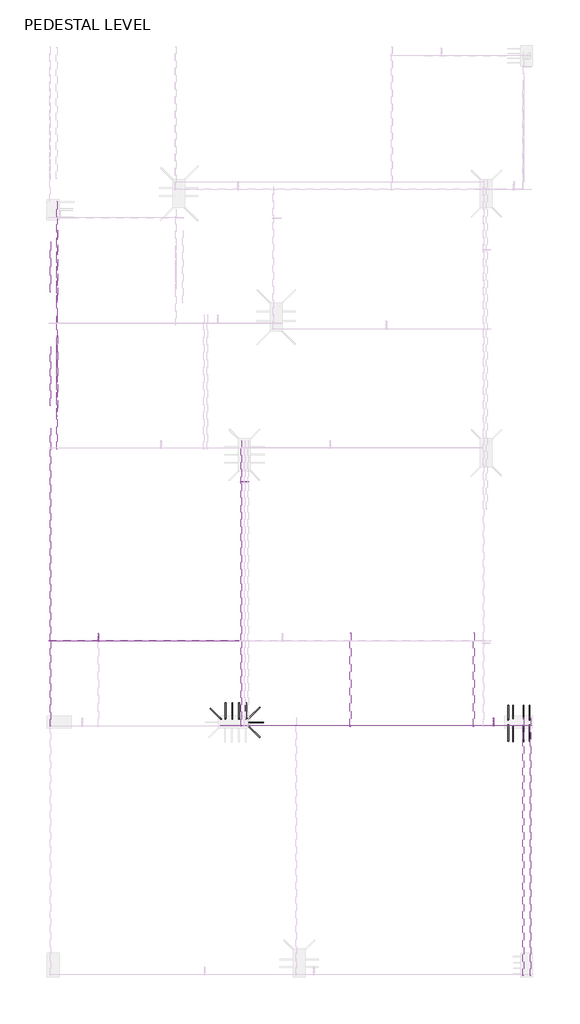
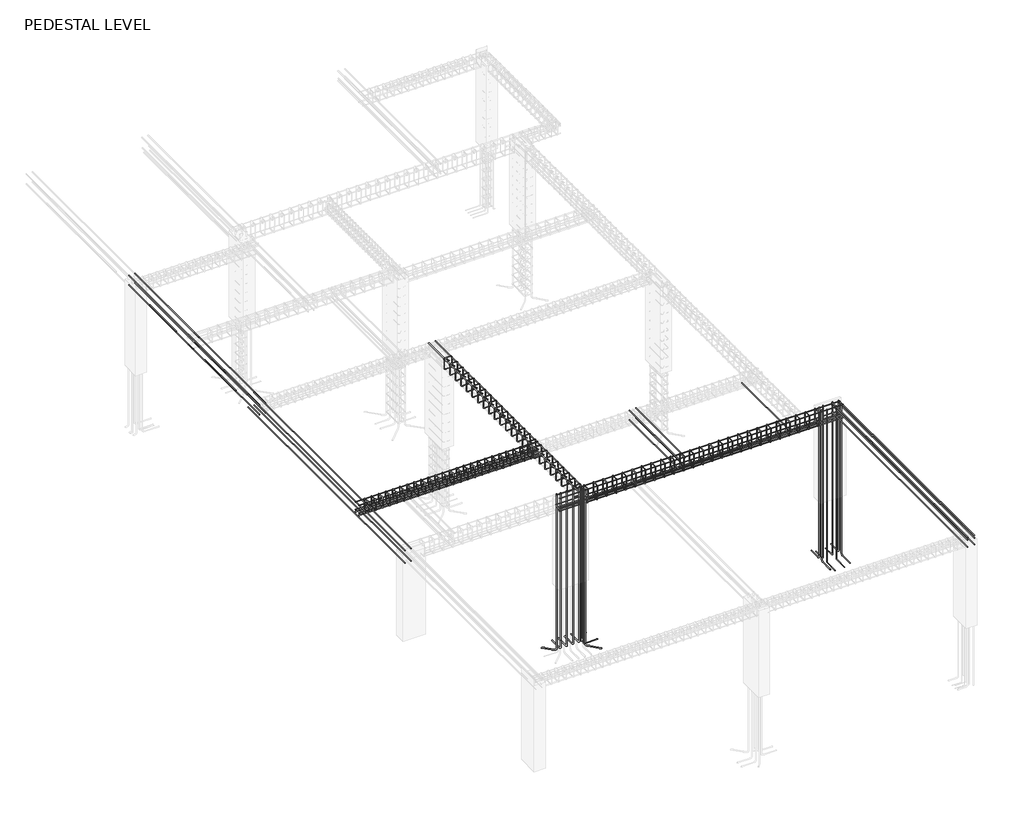
# One storey, part 3 of 8: 35 reinforcing bars.
"""IFC4 building model written with IfcOpenShell, lengths in millimetres."""

from ifc_helpers import new_model, si_unit, point, frame, origin, place, context, project, spatial, polyline, circle_curve, trimmed, segment, composite_curve, source, transform, mapped, element, save
from ifc_brep_helpers import swept_disk

model = new_model("IFC4")

# Units and contexts
model_context = context("Model", 3, world=origin())
ifc_project = project(units=[si_unit("LENGTHUNIT", "METRE", prefix="MILLI")], contexts=[model_context])

# Site, building, storey
site = spatial("IfcSite", under=ifc_project)
building = spatial("IfcBuilding", under=site)
storey = spatial("IfcBuildingStorey", under=building, Name="PEDESTAL LEVEL", Elevation=990.6)

# Reinforcing bars
placement = place(None, origin())
reinforcing_bar_shape = source(origin(), model_context, "Body", "SolidModel", [
    swept_disk(composite_curve([segment(polyline([(153625.7025689, -105009.8007776, 2960.0), (153625.7025689, -105009.8007776, -403.6)]), True, "CONTINUOUS"), segment(trimmed(circle_curve(frame((153625.7025689, -104969.8007776, -403.6), z_axis=(1.0, 0.0, 0.0), x_axis=(0.0, -40.0, 0.0)), 40.0), [point((153625.7025689, -105009.8007776, -403.6))], [point((153625.7025689, -104969.8007776, -443.6))], True, "CARTESIAN"), True, "CONTINUOUS"), segment(polyline([(153625.7025689, -104969.8007776, -443.6), (153625.7025689, -104708.6268212, -443.6)]), True, "CONTINUOUS")], self_intersect=False), 8.0),
])
element("IfcReinforcingBar", 1, at=placement, inside=storey, context=model_context, shape_type="MappedRepresentation", body=[
    mapped(reinforcing_bar_shape, transform((0.0, 0.0, 0.0), x_axis=(1.0, 0.0, 0.0), y_axis=(0.0, 1.0, 0.0), z_axis=(0.0, 0.0, 1.0))),
    mapped(reinforcing_bar_shape, transform((128.9768921, 0.0, 0.0), x_axis=(1.0, 0.0, 0.0), y_axis=(0.0, 1.0, 0.0), z_axis=(0.0, 0.0, 1.0))),
    mapped(reinforcing_bar_shape, transform((257.9537841, 0.0, 0.0), x_axis=(1.0, 0.0, 0.0), y_axis=(0.0, 1.0, 0.0), z_axis=(0.0, 0.0, 1.0))),
    mapped(reinforcing_bar_shape, transform((386.9306762, 0.0, 0.0), x_axis=(1.0, 0.0, 0.0), y_axis=(0.0, 1.0, 0.0), z_axis=(0.0, 0.0, 1.0))),
])
element("IfcReinforcingBar", 2, at=placement, inside=storey, context=model_context, shape_type="SolidModel", body=[
    swept_disk(composite_curve([segment(polyline([(153541.8370351, -105010.3572281, 2960.0), (153541.8370351, -105010.3572281, -403.6)]), True, "CONTINUOUS"), segment(trimmed(circle_curve(frame((153513.5527639, -104982.0729569, -403.6), z_axis=(0.7071067811865475, 0.7071067811865476, 0.0), x_axis=(28.28427120001288, -28.28427119999833, 0.0)), 40.0), [point((153541.8370351, -105010.3572281, -403.6))], [point((153513.5527639, -104982.0729569, -443.6))], True, "CARTESIAN"), True, "CONTINUOUS"), segment(polyline([(153513.5527639, -104982.0729569, -443.6), (153344.8044377, -104813.3246307, -443.6)]), True, "CONTINUOUS")], self_intersect=False), 8.0),
])
element("IfcReinforcingBar", 3, at=placement, inside=storey, context=model_context, shape_type="SolidModel", body=[
    swept_disk(composite_curve([segment(polyline([(154054.8805846, -105009.8007776, 2960.0), (154054.8805846, -105009.8007776, -403.6)]), True, "CONTINUOUS"), segment(trimmed(circle_curve(frame((154083.1648558, -104981.5165063, -403.6), z_axis=(0.7071067811865475, -0.7071067811865476, 0.0), x_axis=(-28.284271199983777, -28.28427129999909, 0.0)), 40.0), [point((154054.8805846, -105009.8007776, -403.6))], [point((154083.1648558, -104981.5165063, -443.6))], True, "CARTESIAN"), True, "CONTINUOUS"), segment(polyline([(154083.1648558, -104981.5165063, -443.6), (154270.4067315, -104794.2746307, -443.6)]), True, "CONTINUOUS")], self_intersect=False), 8.0),
])
element("IfcReinforcingBar", 4, at=placement, inside=storey, context=model_context, shape_type="SolidModel", body=[
    swept_disk(composite_curve([segment(polyline([(154054.3854805, -105141.9056735, 2960.0), (154054.3854805, -105141.9056735, -403.6)]), True, "CONTINUOUS"), segment(trimmed(circle_curve(frame((154082.6697518, -105170.1899448, -403.6), z_axis=(-0.7071067811865475, -0.7071067811865476, 0.0), x_axis=(-28.28427129998454, 28.28427129999909, 0.0)), 40.0), [point((154054.3854805, -105141.9056735, -403.6))], [point((154082.6697518, -105170.1899448, -443.6))], True, "CARTESIAN"), True, "CONTINUOUS"), segment(polyline([(154082.6697518, -105170.1899448, -443.6), (154270.4067315, -105357.9269245, -443.6)]), True, "CONTINUOUS")], self_intersect=False), 8.0),
])
element("IfcReinforcingBar", 5, at=placement, inside=storey, context=model_context, shape_type="SolidModel", body=[
    swept_disk(composite_curve([segment(polyline([(154058.8805846, -105076.4757776, 2960.0), (154058.8805846, -105076.4757776, -423.6)]), True, "CONTINUOUS"), segment(trimmed(circle_curve(frame((154078.8805846, -105076.4757776, -423.6), z_axis=(0.0, -1.0, 0.0), x_axis=(-20.0, 0.0, 0.0)), 20.0), [point((154058.8805846, -105076.4757776, -423.6))], [point((154078.8805846, -105076.4757776, -443.6))], True, "CARTESIAN"), True, "CONTINUOUS"), segment(polyline([(154078.8805846, -105076.4757776, -443.6), (154346.9805846, -105076.4757776, -443.6)]), True, "CONTINUOUS")], self_intersect=False), 4.0),
])
reinforcing_bar_2_shape = source(origin(), model_context, "Body", "SolidModel", [
    swept_disk(composite_curve([segment(polyline([(159353.7369154, -105125.7144861, 2970.0), (159353.7369154, -105125.7144861, -281.3228881)]), True, "CONTINUOUS"), segment(trimmed(circle_curve(frame((159353.7369154, -105165.7144861, -281.3228881), z_axis=(-1.0, 0.0, 0.0), x_axis=(0.0, 40.0, 0.0)), 40.0), [point((159353.7369154, -105125.7144861, -281.3228881))], [point((159353.7369154, -105165.7144861, -321.3228881))], True, "CARTESIAN"), True, "CONTINUOUS"), segment(polyline([(159353.7369154, -105165.7144861, -321.3228881), (159353.7369154, -105430.5144861, -321.3228881)]), True, "CONTINUOUS")], self_intersect=False), 8.0),
])
element("IfcReinforcingBar", 6, at=placement, inside=storey, context=model_context, shape_type="MappedRepresentation", body=[
    mapped(reinforcing_bar_2_shape, transform((0.0, 0.0, 0.0), x_axis=(1.0, 0.0, 0.0), y_axis=(0.0, 1.0, 0.0), z_axis=(0.0, 0.0, 1.0))),
    mapped(reinforcing_bar_2_shape, transform((-404.027417, 0.0, 0.0), x_axis=(1.0, 0.0, 0.0), y_axis=(0.0, 1.0, 0.0), z_axis=(0.0, 0.0, 1.0))),
])
reinforcing_bar_3_shape = source(origin(), model_context, "Body", "SolidModel", [
    swept_disk(composite_curve([segment(polyline([(159353.7369154, -105026.4870691, 2970.0), (159353.7369154, -105026.4870691, -278.4710053)]), True, "CONTINUOUS"), segment(trimmed(circle_curve(frame((159353.7369154, -104986.4870691, -278.4710053), z_axis=(1.0, 0.0, 0.0), x_axis=(0.0, -40.0, 0.0)), 40.0), [point((159353.7369154, -105026.4870691, -278.4710053))], [point((159353.7369154, -104986.4870691, -318.4710053))], True, "CARTESIAN"), True, "CONTINUOUS"), segment(polyline([(159353.7369154, -104986.4870691, -318.4710053), (159353.7369154, -104755.0681161, -318.4710053)]), True, "CONTINUOUS")], self_intersect=False), 8.0),
])
element("IfcReinforcingBar", 7, at=placement, inside=storey, context=model_context, shape_type="MappedRepresentation", body=[
    mapped(reinforcing_bar_3_shape, transform((0.0, 0.0, 0.0), x_axis=(1.0, 0.0, 0.0), y_axis=(0.0, 1.0, 0.0), z_axis=(0.0, 0.0, 1.0))),
    mapped(reinforcing_bar_3_shape, transform((-404.027417, 0.0, 0.0), x_axis=(1.0, 0.0, 0.0), y_axis=(0.0, 1.0, 0.0), z_axis=(0.0, 0.0, 1.0))),
])
reinforcing_bar_4_shape = source(origin(), model_context, "Body", "SolidModel", [
    swept_disk(composite_curve([segment(polyline([(159237.8663807, -105148.4007776, 2970.0), (159237.8663807, -105148.4007776, -348.4618667)]), True, "CONTINUOUS"), segment(trimmed(circle_curve(frame((159237.8663807, -105168.4007776, -348.4618667), z_axis=(-1.0, 0.0, 0.0), x_axis=(0.0, 20.0, 0.0)), 20.0), [point((159237.8663807, -105148.4007776, -348.4618667))], [point((159237.8663807, -105168.4007776, -368.4618667))], True, "CARTESIAN"), True, "CONTINUOUS"), segment(polyline([(159237.8663807, -105168.4007776, -368.4618667), (159237.8663807, -105442.4007776, -368.4618667)]), True, "CONTINUOUS")], self_intersect=False), 4.0),
])
element("IfcReinforcingBar", 8, at=placement, inside=storey, context=model_context, shape_type="MappedRepresentation", body=[
    mapped(reinforcing_bar_4_shape, transform((0.0, 0.0, 0.0), x_axis=(1.0, 0.0, 0.0), y_axis=(0.0, 1.0, 0.0), z_axis=(0.0, 0.0, 1.0))),
    mapped(reinforcing_bar_4_shape, transform((-197.0944443, 0.0, 0.0), x_axis=(1.0, 0.0, 0.0), y_axis=(0.0, 1.0, 0.0), z_axis=(0.0, 0.0, 1.0))),
])
reinforcing_bar_5_shape = source(origin(), model_context, "Body", "SolidModel", [
    swept_disk(composite_curve([segment(polyline([(159237.8663807, -105003.8007776, 2970.0), (159237.8663807, -105003.8007776, -348.4618667)]), True, "CONTINUOUS"), segment(trimmed(circle_curve(frame((159237.8663807, -104983.8007776, -348.4618667), z_axis=(1.0, 0.0, 0.0), x_axis=(0.0, -20.0, 0.0)), 20.0), [point((159237.8663807, -105003.8007776, -348.4618667))], [point((159237.8663807, -104983.8007776, -368.4618667))], True, "CARTESIAN"), True, "CONTINUOUS"), segment(polyline([(159237.8663807, -104983.8007776, -368.4618667), (159237.8663807, -104756.6548318, -368.4618667)]), True, "CONTINUOUS")], self_intersect=False), 4.0),
])
element("IfcReinforcingBar", 9, at=placement, inside=storey, context=model_context, shape_type="MappedRepresentation", body=[
    mapped(reinforcing_bar_5_shape, transform((0.0, 0.0, 0.0), x_axis=(1.0, 0.0, 0.0), y_axis=(0.0, 1.0, 0.0), z_axis=(0.0, 0.0, 1.0))),
    mapped(reinforcing_bar_5_shape, transform((-197.0944443, 0.0, 0.0), x_axis=(1.0, 0.0, 0.0), y_axis=(0.0, 1.0, 0.0), z_axis=(0.0, 0.0, 1.0))),
])
reinforcing_bar_6_shape = source(origin(), model_context, "Body", "SolidModel", [
    swept_disk(composite_curve([segment(polyline([(150331.3521391, -97578.5007776, 2953.0710678), (150331.3521391, -95276.3007776, 2953.0710678)]), True, "CONTINUOUS")], self_intersect=False), 6.0),
])
element("IfcReinforcingBar", 10, at=placement, inside=storey, context=model_context, shape_type="MappedRepresentation", body=[
    mapped(reinforcing_bar_6_shape, transform((0.0, 0.0, 0.0), x_axis=(1.0, 0.0, 0.0), y_axis=(0.0, 1.0, 0.0), z_axis=(0.0, 0.0, 1.0))),
    mapped(reinforcing_bar_6_shape, transform((124.7421356, 0.0, 0.0), x_axis=(1.0, 0.0, 0.0), y_axis=(0.0, 1.0, 0.0), z_axis=(0.0, 0.0, 1.0))),
])
reinforcing_bar_7_shape = source(origin(), model_context, "Body", "SolidModel", [
    swept_disk(composite_curve([segment(polyline([(150331.3521391, -97578.5007776, 2742.1289322), (150331.3521391, -95276.3007776, 2742.1289322)]), True, "CONTINUOUS")], self_intersect=False), 6.0),
])
element("IfcReinforcingBar", 11, at=placement, inside=storey, context=model_context, shape_type="MappedRepresentation", body=[
    mapped(reinforcing_bar_7_shape, transform((0.0, 0.0, 0.0), x_axis=(1.0, 0.0, 0.0), y_axis=(0.0, 1.0, 0.0), z_axis=(0.0, 0.0, 1.0))),
    mapped(reinforcing_bar_7_shape, transform((124.7421356, 0.0, 0.0), x_axis=(1.0, 0.0, 0.0), y_axis=(0.0, 1.0, 0.0), z_axis=(0.0, 0.0, 1.0))),
])
element("IfcReinforcingBar", 12, at=placement, inside=storey, context=model_context, shape_type="SolidModel", body=[
    swept_disk(composite_curve([segment(polyline([(150328.4232069, -96983.6572557, 2771.4), (150328.4232069, -96032.524691, 2771.4)]), True, "CONTINUOUS")], self_intersect=False), 6.0),
])
element("IfcReinforcingBar", 13, at=placement, inside=storey, context=model_context, shape_type="SolidModel", body=[
    swept_disk(composite_curve([segment(polyline([(150459.0232069, -97175.4075722, 2771.4), (150459.0232069, -95820.3079229, 2771.4)]), True, "CONTINUOUS")], self_intersect=False), 6.0),
])
reinforcing_bar_8_shape = source(origin(), model_context, "Body", "SolidModel", [
    swept_disk(composite_curve([segment(polyline([(150331.3521391, -99940.7007776, 2953.0710678), (150331.3521391, -97409.9007776, 2953.0710678)]), True, "CONTINUOUS")], self_intersect=False), 6.0),
])
element("IfcReinforcingBar", 14, at=placement, inside=storey, context=model_context, shape_type="MappedRepresentation", body=[
    mapped(reinforcing_bar_8_shape, transform((0.0, 0.0, 0.0), x_axis=(1.0, 0.0, 0.0), y_axis=(0.0, 1.0, 0.0), z_axis=(0.0, 0.0, 1.0))),
    mapped(reinforcing_bar_8_shape, transform((124.7421356, 0.0, 0.0), x_axis=(1.0, 0.0, 0.0), y_axis=(0.0, 1.0, 0.0), z_axis=(0.0, 0.0, 1.0))),
])
reinforcing_bar_9_shape = source(origin(), model_context, "Body", "SolidModel", [
    swept_disk(composite_curve([segment(polyline([(150331.3521391, -99940.7007776, 2742.1289322), (150331.3521391, -97409.9007776, 2742.1289322)]), True, "CONTINUOUS")], self_intersect=False), 6.0),
])
element("IfcReinforcingBar", 15, at=placement, inside=storey, context=model_context, shape_type="MappedRepresentation", body=[
    mapped(reinforcing_bar_9_shape, transform((0.0, 0.0, 0.0), x_axis=(1.0, 0.0, 0.0), y_axis=(0.0, 1.0, 0.0), z_axis=(0.0, 0.0, 1.0))),
    mapped(reinforcing_bar_9_shape, transform((124.7421356, 0.0, 0.0), x_axis=(1.0, 0.0, 0.0), y_axis=(0.0, 1.0, 0.0), z_axis=(0.0, 0.0, 1.0))),
])
element("IfcReinforcingBar", 16, at=placement, inside=storey, context=model_context, shape_type="SolidModel", body=[
    swept_disk(composite_curve([segment(polyline([(150328.4232069, -99117.2572557, 2771.4), (150328.4232069, -98013.7246916, 2771.4)]), True, "CONTINUOUS")], self_intersect=False), 6.0),
])
element("IfcReinforcingBar", 17, at=placement, inside=storey, context=model_context, shape_type="SolidModel", body=[
    swept_disk(composite_curve([segment(polyline([(150459.0232069, -99316.7901782, 2771.4), (150459.0232069, -97803.9257644, 2771.4)]), True, "CONTINUOUS")], self_intersect=False), 6.0),
])
reinforcing_bar_10_shape = source(origin(), model_context, "Body", "SolidModel", [
    swept_disk(composite_curve([segment(polyline([(159236.7521391, -109846.7007776, 2953.0710678), (159236.7521391, -104991.8007776, 2953.0710678)]), True, "CONTINUOUS")], self_intersect=False), 6.0),
])
element("IfcReinforcingBar", 18, at=placement, inside=storey, context=model_context, shape_type="MappedRepresentation", body=[
    mapped(reinforcing_bar_10_shape, transform((0.0, 0.0, 0.0), x_axis=(1.0, 0.0, 0.0), y_axis=(0.0, 1.0, 0.0), z_axis=(0.0, 0.0, 1.0))),
    mapped(reinforcing_bar_10_shape, transform((134.7421356, 0.0, 0.0), x_axis=(1.0, 0.0, 0.0), y_axis=(0.0, 1.0, 0.0), z_axis=(0.0, 0.0, 1.0))),
])
reinforcing_bar_11_shape = source(origin(), model_context, "Body", "SolidModel", [
    swept_disk(composite_curve([segment(polyline([(159374.4232069, -109846.7007776, 2749.2), (159374.4232069, -104991.8007776, 2749.2)]), True, "CONTINUOUS")], self_intersect=False), 6.0),
])
element("IfcReinforcingBar", 19, at=placement, inside=storey, context=model_context, shape_type="MappedRepresentation", body=[
    mapped(reinforcing_bar_11_shape, transform((0.0, 0.0, 0.0), x_axis=(1.0, 0.0, 0.0), y_axis=(0.0, 1.0, 0.0), z_axis=(0.0, 0.0, 1.0))),
    mapped(reinforcing_bar_11_shape, transform((-140.6, 0.0, 0.0), x_axis=(1.0, 0.0, 0.0), y_axis=(0.0, 1.0, 0.0), z_axis=(0.0, 0.0, 1.0))),
])
reinforcing_bar_12_shape = source(origin(), model_context, "Body", "SolidModel", [
    swept_disk(composite_curve([segment(polyline([(159233.8232069, -109846.7007776, 2896.5439131), (159233.8232069, -104991.8007776, 2896.5439131)]), True, "CONTINUOUS")], self_intersect=False), 6.0),
])
element("IfcReinforcingBar", 20, at=placement, inside=storey, context=model_context, shape_type="MappedRepresentation", body=[
    mapped(reinforcing_bar_12_shape, transform((0.0, 0.0, 0.0), x_axis=(1.0, 0.0, 0.0), y_axis=(0.0, 1.0, 0.0), z_axis=(0.0, 0.0, 1.0))),
    mapped(reinforcing_bar_12_shape, transform((140.6, 0.0, 0.0), x_axis=(1.0, 0.0, 0.0), y_axis=(0.0, 1.0, 0.0), z_axis=(0.0, 0.0, 1.0))),
])
reinforcing_bar_13_shape = source(origin(), model_context, "Body", "SolidModel", [
    swept_disk(composite_curve([segment(polyline([(150507.0232063, -103455.5119243, 2895.7954185), (150507.0232063, -103519.8586414, 2960.1421356)]), True, "CONTINUOUS"), segment(trimmed(circle_curve(frame((150507.0232063, -103534.000777, 2946.0), z_axis=(1.0, 0.0, 0.0), x_axis=(0.0, 14.142135599991889, 14.142135600000074)), 20.0), [point((150507.0232063, -103519.8586414, 2960.1421356))], [point((150507.0232063, -103554.000777, 2946.0))], True, "CARTESIAN"), True, "CONTINUOUS"), segment(polyline([(150507.0232063, -103554.000777, 2946.0), (150507.0232063, -103554.000777, 2749.2)]), True, "CONTINUOUS"), segment(trimmed(circle_curve(frame((150507.0232063, -103534.000777, 2749.2), z_axis=(1.0, 0.0, 0.0), x_axis=(0.0, -20.0, 0.0)), 20.0), [point((150507.0232063, -103554.000777, 2749.2))], [point((150507.0232063, -103534.000777, 2729.2))], True, "CARTESIAN"), True, "CONTINUOUS"), segment(polyline([(150507.0232063, -103534.000777, 2729.2), (150507.0232063, -103423.400777, 2729.2)]), True, "CONTINUOUS"), segment(trimmed(circle_curve(frame((150506.3479159, -103423.400777, 2749.1885963), z_axis=(0.9994298160123042, 0.0, 0.033764520811226544), x_axis=(0.6752903999877162, 0.0, -19.988596300000154)), 20.0), [point((150507.0232063, -103423.400777, 2729.2))], [point((150506.3479159, -103403.400777, 2749.1885963))], True, "CARTESIAN"), True, "CONTINUOUS"), segment(polyline([(150506.3479159, -103403.400777, 2749.1885963), (150499.6984967, -103403.400777, 2946.0114037)]), True, "CONTINUOUS"), segment(trimmed(circle_curve(frame((150499.6984967, -103423.400777, 2946.0114037), z_axis=(0.9994298160123042, 0.0, 0.033764520811226544), x_axis=(0.0, 20.0, 0.0)), 20.0), [point((150499.6984967, -103403.400777, 2946.0114037))], [point((150499.0232063, -103423.400777, 2966.0))], True, "CARTESIAN"), True, "CONTINUOUS"), segment(polyline([(150499.0232063, -103423.400777, 2966.0), (150499.0232063, -103534.000777, 2966.0)]), True, "CONTINUOUS"), segment(trimmed(circle_curve(frame((150499.0232063, -103534.000777, 2946.0), z_axis=(1.0, 0.0, 0.0), x_axis=(0.0, 0.0, 20.0)), 20.0), [point((150499.0232063, -103534.000777, 2966.0))], [point((150499.0232063, -103548.1429126, 2931.8578644))], True, "CARTESIAN"), True, "CONTINUOUS"), segment(polyline([(150499.0232063, -103548.1429126, 2931.8578644), (150499.0232063, -103483.7961955, 2867.5111473)]), True, "CONTINUOUS")], self_intersect=False), 4.0),
])
element("IfcReinforcingBar", 21, at=placement, inside=storey, context=model_context, shape_type="MappedRepresentation", body=[
    mapped(reinforcing_bar_13_shape, transform((0.0, 0.0, 0.0), x_axis=(1.0, 0.0, 0.0), y_axis=(0.0, 1.0, 0.0), z_axis=(0.0, 0.0, 1.0))),
    mapped(reinforcing_bar_13_shape, transform((146.2285817, 0.0, 0.0), x_axis=(1.0, 0.0, 0.0), y_axis=(0.0, 1.0, 0.0), z_axis=(0.0, 0.0, 1.0))),
    mapped(reinforcing_bar_13_shape, transform((292.4571634, 0.0, 0.0), x_axis=(1.0, 0.0, 0.0), y_axis=(0.0, 1.0, 0.0), z_axis=(0.0, 0.0, 1.0))),
    mapped(reinforcing_bar_13_shape, transform((438.6857451, 0.0, 0.0), x_axis=(1.0, 0.0, 0.0), y_axis=(0.0, 1.0, 0.0), z_axis=(0.0, 0.0, 1.0))),
    mapped(reinforcing_bar_13_shape, transform((584.9143268, 0.0, 0.0), x_axis=(1.0, 0.0, 0.0), y_axis=(0.0, 1.0, 0.0), z_axis=(0.0, 0.0, 1.0))),
    mapped(reinforcing_bar_13_shape, transform((731.1429084, 0.0, 0.0), x_axis=(1.0, 0.0, 0.0), y_axis=(0.0, 1.0, 0.0), z_axis=(0.0, 0.0, 1.0))),
    mapped(reinforcing_bar_13_shape, transform((877.3714901, 0.0, 0.0), x_axis=(1.0, 0.0, 0.0), y_axis=(0.0, 1.0, 0.0), z_axis=(0.0, 0.0, 1.0))),
    mapped(reinforcing_bar_13_shape, transform((1023.6000718, 0.0, 0.0), x_axis=(1.0, 0.0, 0.0), y_axis=(0.0, 1.0, 0.0), z_axis=(0.0, 0.0, 1.0))),
    mapped(reinforcing_bar_13_shape, transform((1169.8286535, 0.0, 0.0), x_axis=(1.0, 0.0, 0.0), y_axis=(0.0, 1.0, 0.0), z_axis=(0.0, 0.0, 1.0))),
    mapped(reinforcing_bar_13_shape, transform((1316.0572352, 0.0, 0.0), x_axis=(1.0, 0.0, 0.0), y_axis=(0.0, 1.0, 0.0), z_axis=(0.0, 0.0, 1.0))),
    mapped(reinforcing_bar_13_shape, transform((1462.2858169, 0.0, 0.0), x_axis=(1.0, 0.0, 0.0), y_axis=(0.0, 1.0, 0.0), z_axis=(0.0, 0.0, 1.0))),
    mapped(reinforcing_bar_13_shape, transform((1608.5143986, 0.0, 0.0), x_axis=(1.0, 0.0, 0.0), y_axis=(0.0, 1.0, 0.0), z_axis=(0.0, 0.0, 1.0))),
    mapped(reinforcing_bar_13_shape, transform((1754.7429803, 0.0, 0.0), x_axis=(1.0, 0.0, 0.0), y_axis=(0.0, 1.0, 0.0), z_axis=(0.0, 0.0, 1.0))),
    mapped(reinforcing_bar_13_shape, transform((1900.971562, 0.0, 0.0), x_axis=(1.0, 0.0, 0.0), y_axis=(0.0, 1.0, 0.0), z_axis=(0.0, 0.0, 1.0))),
    mapped(reinforcing_bar_13_shape, transform((2047.2001437, 0.0, 0.0), x_axis=(1.0, 0.0, 0.0), y_axis=(0.0, 1.0, 0.0), z_axis=(0.0, 0.0, 1.0))),
    mapped(reinforcing_bar_13_shape, transform((2193.4287253, 0.0, 0.0), x_axis=(1.0, 0.0, 0.0), y_axis=(0.0, 1.0, 0.0), z_axis=(0.0, 0.0, 1.0))),
    mapped(reinforcing_bar_13_shape, transform((2339.657307, 0.0, 0.0), x_axis=(1.0, 0.0, 0.0), y_axis=(0.0, 1.0, 0.0), z_axis=(0.0, 0.0, 1.0))),
    mapped(reinforcing_bar_13_shape, transform((2485.8858887, 0.0, 0.0), x_axis=(1.0, 0.0, 0.0), y_axis=(0.0, 1.0, 0.0), z_axis=(0.0, 0.0, 1.0))),
    mapped(reinforcing_bar_13_shape, transform((2632.1144704, 0.0, 0.0), x_axis=(1.0, 0.0, 0.0), y_axis=(0.0, 1.0, 0.0), z_axis=(0.0, 0.0, 1.0))),
    mapped(reinforcing_bar_13_shape, transform((2778.3430521, 0.0, 0.0), x_axis=(1.0, 0.0, 0.0), y_axis=(0.0, 1.0, 0.0), z_axis=(0.0, 0.0, 1.0))),
    mapped(reinforcing_bar_13_shape, transform((2924.5716338, 0.0, 0.0), x_axis=(1.0, 0.0, 0.0), y_axis=(0.0, 1.0, 0.0), z_axis=(0.0, 0.0, 1.0))),
    mapped(reinforcing_bar_13_shape, transform((3070.8002155, 0.0, 0.0), x_axis=(1.0, 0.0, 0.0), y_axis=(0.0, 1.0, 0.0), z_axis=(0.0, 0.0, 1.0))),
    mapped(reinforcing_bar_13_shape, transform((3217.0287972, 0.0, 0.0), x_axis=(1.0, 0.0, 0.0), y_axis=(0.0, 1.0, 0.0), z_axis=(0.0, 0.0, 1.0))),
    mapped(reinforcing_bar_13_shape, transform((3363.2573789, 0.0, 0.0), x_axis=(1.0, 0.0, 0.0), y_axis=(0.0, 1.0, 0.0), z_axis=(0.0, 0.0, 1.0))),
])
reinforcing_bar_14_shape = source(origin(), model_context, "Body", "SolidModel", [
    swept_disk(composite_curve([segment(polyline([(150304.4232069, -103416.3297092, 2953.0710678), (154072.8805846, -103416.3297092, 2953.0710678)]), True, "CONTINUOUS")], self_intersect=False), 6.0),
])
element("IfcReinforcingBar", 22, at=placement, inside=storey, context=model_context, shape_type="MappedRepresentation", body=[
    mapped(reinforcing_bar_14_shape, transform((0.0, 0.0, 0.0), x_axis=(1.0, 0.0, 0.0), y_axis=(0.0, 1.0, 0.0), z_axis=(0.0, 0.0, 1.0))),
    mapped(reinforcing_bar_14_shape, transform((0.0, -124.7421356, 0.0), x_axis=(1.0, 0.0, 0.0), y_axis=(0.0, 1.0, 0.0), z_axis=(0.0, 0.0, 1.0))),
])
reinforcing_bar_15_shape = source(origin(), model_context, "Body", "SolidModel", [
    swept_disk(composite_curve([segment(polyline([(150304.4232069, -103541.0718448, 2742.1289322), (154072.8805846, -103541.0718448, 2742.1289322)]), True, "CONTINUOUS")], self_intersect=False), 6.0),
])
element("IfcReinforcingBar", 23, at=placement, inside=storey, context=model_context, shape_type="MappedRepresentation", body=[
    mapped(reinforcing_bar_15_shape, transform((0.0, 0.0, 0.0), x_axis=(1.0, 0.0, 0.0), y_axis=(0.0, 1.0, 0.0), z_axis=(0.0, 0.0, 1.0))),
    mapped(reinforcing_bar_15_shape, transform((0.0, 124.7421356, 0.0), x_axis=(1.0, 0.0, 0.0), y_axis=(0.0, 1.0, 0.0), z_axis=(0.0, 0.0, 1.0))),
])
reinforcing_bar_16_shape = source(origin(), model_context, "Body", "SolidModel", [
    swept_disk(composite_curve([segment(polyline([(150304.4232069, -103544.000777, 2791.7182247), (154072.8805846, -103544.000777, 2791.7182247)]), True, "CONTINUOUS")], self_intersect=False), 6.0),
])
element("IfcReinforcingBar", 24, at=placement, inside=storey, context=model_context, shape_type="MappedRepresentation", body=[
    mapped(reinforcing_bar_16_shape, transform((0.0, 0.0, 0.0), x_axis=(1.0, 0.0, 0.0), y_axis=(0.0, 1.0, 0.0), z_axis=(0.0, 0.0, 1.0))),
    mapped(reinforcing_bar_16_shape, transform((0.0, 127.6710678, 0.0), x_axis=(1.0, 0.0, 0.0), y_axis=(0.0, 1.0, 0.0), z_axis=(0.0, 0.0, 1.0))),
])
reinforcing_bar_17_shape = source(origin(), model_context, "Body", "SolidModel", [
    swept_disk(composite_curve([segment(polyline([(150331.3521391, -105150.4007776, 2943.0710678), (150331.3521391, -99543.5007776, 2943.0710678)]), True, "CONTINUOUS")], self_intersect=False), 6.0),
])
element("IfcReinforcingBar", 25, at=placement, inside=storey, context=model_context, shape_type="MappedRepresentation", body=[
    mapped(reinforcing_bar_17_shape, transform((0.0, 0.0, 0.0), x_axis=(1.0, 0.0, 0.0), y_axis=(0.0, 1.0, 0.0), z_axis=(0.0, 0.0, 1.0))),
    mapped(reinforcing_bar_17_shape, transform((124.7421356, 0.0, 0.0), x_axis=(1.0, 0.0, 0.0), y_axis=(0.0, 1.0, 0.0), z_axis=(0.0, 0.0, 1.0))),
])
reinforcing_bar_18_shape = source(origin(), model_context, "Body", "SolidModel", [
    swept_disk(composite_curve([segment(polyline([(150331.3521391, -105150.4007776, 2665.826012), (150331.3521391, -99543.5007776, 2665.826012)]), True, "CONTINUOUS")], self_intersect=False), 6.0),
])
element("IfcReinforcingBar", 26, at=placement, inside=storey, context=model_context, shape_type="MappedRepresentation", body=[
    mapped(reinforcing_bar_18_shape, transform((0.0, 0.0, 0.0), x_axis=(1.0, 0.0, 0.0), y_axis=(0.0, 1.0, 0.0), z_axis=(0.0, 0.0, 1.0))),
    mapped(reinforcing_bar_18_shape, transform((124.7421356, 0.0, 0.0), x_axis=(1.0, 0.0, 0.0), y_axis=(0.0, 1.0, 0.0), z_axis=(0.0, 0.0, 1.0))),
])
reinforcing_bar_19_shape = source(origin(), model_context, "Body", "SolidModel", [
    swept_disk(composite_curve([segment(polyline([(154006.7694373, -100357.7007776, 2895.7954185), (153942.4227202, -100357.7007776, 2960.1421356)]), True, "CONTINUOUS"), segment(trimmed(circle_curve(frame((153928.2805846, -100357.7007776, 2946.0), z_axis=(0.0, -1.0, 0.0), x_axis=(14.14213560000644, 0.0, 14.142135600000074)), 20.0), [point((153942.4227202, -100357.7007776, 2960.1421356))], [point((153908.2805846, -100357.7007776, 2946.0))], True, "CARTESIAN"), True, "CONTINUOUS"), segment(polyline([(153908.2805846, -100357.7007776, 2946.0), (153908.2805846, -100357.7007776, 2749.2)]), True, "CONTINUOUS"), segment(trimmed(circle_curve(frame((153928.2805846, -100357.7007776, 2749.2), z_axis=(0.0, -1.0, 0.0), x_axis=(-20.0, 0.0, 0.0)), 20.0), [point((153908.2805846, -100357.7007776, 2749.2))], [point((153928.2805846, -100357.7007776, 2729.2))], True, "CARTESIAN"), True, "CONTINUOUS"), segment(polyline([(153928.2805846, -100357.7007776, 2729.2), (154048.8805846, -100357.7007776, 2729.2)]), True, "CONTINUOUS"), segment(trimmed(circle_curve(frame((154048.8805846, -100357.0254872, 2749.1885963), z_axis=(0.0, -0.9994298160123042, 0.03376452081122655), x_axis=(0.0, -0.6752904000022681, -19.988596300000154)), 20.0), [point((154048.8805846, -100357.7007776, 2729.2))], [point((154068.8805846, -100357.0254872, 2749.1885963))], True, "CARTESIAN"), True, "CONTINUOUS"), segment(polyline([(154068.8805846, -100357.0254872, 2749.1885963), (154068.8805846, -100350.376068, 2946.0114037)]), True, "CONTINUOUS"), segment(trimmed(circle_curve(frame((154048.8805846, -100350.376068, 2946.0114037), z_axis=(0.0, -0.9994298160123042, 0.03376452081122655), x_axis=(20.0, 0.0, 0.0)), 20.0), [point((154068.8805846, -100350.376068, 2946.0114037))], [point((154048.8805846, -100349.7007776, 2966.0))], True, "CARTESIAN"), True, "CONTINUOUS"), segment(polyline([(154048.8805846, -100349.7007776, 2966.0), (153928.2805846, -100349.7007776, 2966.0)]), True, "CONTINUOUS"), segment(trimmed(circle_curve(frame((153928.2805846, -100349.7007776, 2946.0), z_axis=(0.0, -1.0, 0.0), x_axis=(0.0, 0.0, 20.0)), 20.0), [point((153928.2805846, -100349.7007776, 2966.0))], [point((153914.138449, -100349.7007776, 2931.8578644))], True, "CARTESIAN"), True, "CONTINUOUS"), segment(polyline([(153914.138449, -100349.7007776, 2931.8578644), (153978.485166, -100349.7007776, 2867.5111473)]), True, "CONTINUOUS")], self_intersect=False), 4.0),
])
element("IfcReinforcingBar", 27, at=placement, inside=storey, context=model_context, shape_type="MappedRepresentation", body=[
    mapped(reinforcing_bar_19_shape, transform((0.0, 0.0, 0.0), x_axis=(1.0, 0.0, 0.0), y_axis=(0.0, 1.0, 0.0), z_axis=(0.0, 0.0, 1.0))),
    mapped(reinforcing_bar_19_shape, transform((0.0, -199.9173913, 0.0), x_axis=(1.0, 0.0, 0.0), y_axis=(0.0, 1.0, 0.0), z_axis=(0.0, 0.0, 1.0))),
    mapped(reinforcing_bar_19_shape, transform((0.0, -399.8347826, 0.0), x_axis=(1.0, 0.0, 0.0), y_axis=(0.0, 1.0, 0.0), z_axis=(0.0, 0.0, 1.0))),
    mapped(reinforcing_bar_19_shape, transform((0.0, -599.7521739, 0.0), x_axis=(1.0, 0.0, 0.0), y_axis=(0.0, 1.0, 0.0), z_axis=(0.0, 0.0, 1.0))),
    mapped(reinforcing_bar_19_shape, transform((0.0, -799.6695652, 0.0), x_axis=(1.0, 0.0, 0.0), y_axis=(0.0, 1.0, 0.0), z_axis=(0.0, 0.0, 1.0))),
    mapped(reinforcing_bar_19_shape, transform((0.0, -999.5869565, 0.0), x_axis=(1.0, 0.0, 0.0), y_axis=(0.0, 1.0, 0.0), z_axis=(0.0, 0.0, 1.0))),
    mapped(reinforcing_bar_19_shape, transform((0.0, -1199.5043478, 0.0), x_axis=(1.0, 0.0, 0.0), y_axis=(0.0, 1.0, 0.0), z_axis=(0.0, 0.0, 1.0))),
    mapped(reinforcing_bar_19_shape, transform((0.0, -1399.4217391, 0.0), x_axis=(1.0, 0.0, 0.0), y_axis=(0.0, 1.0, 0.0), z_axis=(0.0, 0.0, 1.0))),
    mapped(reinforcing_bar_19_shape, transform((0.0, -1599.3391304, 0.0), x_axis=(1.0, 0.0, 0.0), y_axis=(0.0, 1.0, 0.0), z_axis=(0.0, 0.0, 1.0))),
    mapped(reinforcing_bar_19_shape, transform((0.0, -1799.2565217, 0.0), x_axis=(1.0, 0.0, 0.0), y_axis=(0.0, 1.0, 0.0), z_axis=(0.0, 0.0, 1.0))),
    mapped(reinforcing_bar_19_shape, transform((0.0, -1999.173913, 0.0), x_axis=(1.0, 0.0, 0.0), y_axis=(0.0, 1.0, 0.0), z_axis=(0.0, 0.0, 1.0))),
    mapped(reinforcing_bar_19_shape, transform((0.0, -2199.0913043, 0.0), x_axis=(1.0, 0.0, 0.0), y_axis=(0.0, 1.0, 0.0), z_axis=(0.0, 0.0, 1.0))),
    mapped(reinforcing_bar_19_shape, transform((0.0, -2399.0086957, 0.0), x_axis=(1.0, 0.0, 0.0), y_axis=(0.0, 1.0, 0.0), z_axis=(0.0, 0.0, 1.0))),
    mapped(reinforcing_bar_19_shape, transform((0.0, -2598.926087, 0.0), x_axis=(1.0, 0.0, 0.0), y_axis=(0.0, 1.0, 0.0), z_axis=(0.0, 0.0, 1.0))),
    mapped(reinforcing_bar_19_shape, transform((0.0, -2798.8434783, 0.0), x_axis=(1.0, 0.0, 0.0), y_axis=(0.0, 1.0, 0.0), z_axis=(0.0, 0.0, 1.0))),
    mapped(reinforcing_bar_19_shape, transform((0.0, -2998.7608696, 0.0), x_axis=(1.0, 0.0, 0.0), y_axis=(0.0, 1.0, 0.0), z_axis=(0.0, 0.0, 1.0))),
    mapped(reinforcing_bar_19_shape, transform((0.0, -3198.6782609, 0.0), x_axis=(1.0, 0.0, 0.0), y_axis=(0.0, 1.0, 0.0), z_axis=(0.0, 0.0, 1.0))),
    mapped(reinforcing_bar_19_shape, transform((0.0, -3398.5956522, 0.0), x_axis=(1.0, 0.0, 0.0), y_axis=(0.0, 1.0, 0.0), z_axis=(0.0, 0.0, 1.0))),
    mapped(reinforcing_bar_19_shape, transform((0.0, -3598.5130435, 0.0), x_axis=(1.0, 0.0, 0.0), y_axis=(0.0, 1.0, 0.0), z_axis=(0.0, 0.0, 1.0))),
    mapped(reinforcing_bar_19_shape, transform((0.0, -3798.4304348, 0.0), x_axis=(1.0, 0.0, 0.0), y_axis=(0.0, 1.0, 0.0), z_axis=(0.0, 0.0, 1.0))),
    mapped(reinforcing_bar_19_shape, transform((0.0, -3998.3478261, 0.0), x_axis=(1.0, 0.0, 0.0), y_axis=(0.0, 1.0, 0.0), z_axis=(0.0, 0.0, 1.0))),
    mapped(reinforcing_bar_19_shape, transform((0.0, -4198.2652174, 0.0), x_axis=(1.0, 0.0, 0.0), y_axis=(0.0, 1.0, 0.0), z_axis=(0.0, 0.0, 1.0))),
    mapped(reinforcing_bar_19_shape, transform((0.0, -4398.1826087, 0.0), x_axis=(1.0, 0.0, 0.0), y_axis=(0.0, 1.0, 0.0), z_axis=(0.0, 0.0, 1.0))),
    mapped(reinforcing_bar_19_shape, transform((0.0, -4598.1, 0.0), x_axis=(1.0, 0.0, 0.0), y_axis=(0.0, 1.0, 0.0), z_axis=(0.0, 0.0, 1.0))),
])
reinforcing_bar_20_shape = source(origin(), model_context, "Body", "SolidModel", [
    swept_disk(composite_curve([segment(polyline([(154055.9516524, -99782.1007776, 2953.0710678), (154055.9516524, -105150.4007776, 2953.0710678)]), True, "CONTINUOUS")], self_intersect=False), 6.0),
])
element("IfcReinforcingBar", 28, at=placement, inside=storey, context=model_context, shape_type="MappedRepresentation", body=[
    mapped(reinforcing_bar_20_shape, transform((0.0, 0.0, 0.0), x_axis=(1.0, 0.0, 0.0), y_axis=(0.0, 1.0, 0.0), z_axis=(0.0, 0.0, 1.0))),
    mapped(reinforcing_bar_20_shape, transform((-134.7421356, 0.0, 0.0), x_axis=(1.0, 0.0, 0.0), y_axis=(0.0, 1.0, 0.0), z_axis=(0.0, 0.0, 1.0))),
])
reinforcing_bar_21_shape = source(origin(), model_context, "Body", "SolidModel", [
    swept_disk(composite_curve([segment(polyline([(156113.9442747, -103391.6007776, 2953.0710678), (156113.9442747, -105160.4007776, 2953.0710678)]), True, "CONTINUOUS")], self_intersect=False), 6.0),
])
element("IfcReinforcingBar", 29, at=placement, inside=storey, context=model_context, shape_type="MappedRepresentation", body=[
    mapped(reinforcing_bar_21_shape, transform((0.0, 0.0, 0.0), x_axis=(1.0, 0.0, 0.0), y_axis=(0.0, 1.0, 0.0), z_axis=(0.0, 0.0, 1.0))),
    mapped(reinforcing_bar_21_shape, transform((-134.7421356, 0.0, 0.0), x_axis=(1.0, 0.0, 0.0), y_axis=(0.0, 1.0, 0.0), z_axis=(0.0, 0.0, 1.0))),
])
reinforcing_bar_22_shape = source(origin(), model_context, "Body", "SolidModel", [
    swept_disk(composite_curve([segment(polyline([(155979.2021391, -103391.6007776, 2742.1289322), (155979.2021391, -105160.4007776, 2742.1289322)]), True, "CONTINUOUS")], self_intersect=False), 6.0),
])
element("IfcReinforcingBar", 30, at=placement, inside=storey, context=model_context, shape_type="MappedRepresentation", body=[
    mapped(reinforcing_bar_22_shape, transform((0.0, 0.0, 0.0), x_axis=(1.0, 0.0, 0.0), y_axis=(0.0, 1.0, 0.0), z_axis=(0.0, 0.0, 1.0))),
    mapped(reinforcing_bar_22_shape, transform((134.7421356, 0.0, 0.0), x_axis=(1.0, 0.0, 0.0), y_axis=(0.0, 1.0, 0.0), z_axis=(0.0, 0.0, 1.0))),
])
element("IfcReinforcingBar", 31, at=placement, inside=storey, context=model_context, shape_type="SolidModel", body=[
    swept_disk(composite_curve([segment(polyline([(158303.6497425, -103391.6007776, 2739.2), (158303.6497425, -105160.4007776, 2739.2)]), True, "CONTINUOUS")], self_intersect=False), 6.0),
])
reinforcing_bar_23_shape = source(origin(), model_context, "Body", "SolidModel", [
    swept_disk(composite_curve([segment(polyline([(154108.8805846, -105094.2896303, 2723.2045815), (154108.8805846, -105029.9429132, 2658.8578644)]), True, "CONTINUOUS"), segment(trimmed(circle_curve(frame((154108.8805846, -105015.8007776, 2673.0), z_axis=(1.0, 0.0, 0.0), x_axis=(0.0, -14.142135599991889, -14.142135600000074)), 20.0), [point((154108.8805846, -105029.9429132, 2658.8578644))], [point((154108.8805846, -104995.8007776, 2673.0))], True, "CARTESIAN"), True, "CONTINUOUS"), segment(polyline([(154108.8805846, -104995.8007776, 2673.0), (154108.8805846, -104995.8007776, 2936.0)]), True, "CONTINUOUS"), segment(trimmed(circle_curve(frame((154108.8805846, -105015.8007776, 2936.0), z_axis=(1.0, 0.0, 0.0), x_axis=(0.0, 20.0, 0.0)), 20.0), [point((154108.8805846, -104995.8007776, 2936.0))], [point((154108.8805846, -105015.8007776, 2956.0))], True, "CARTESIAN"), True, "CONTINUOUS"), segment(polyline([(154108.8805846, -105015.8007776, 2956.0), (154108.8805846, -105126.4007776, 2956.0)]), True, "CONTINUOUS"), segment(trimmed(circle_curve(frame((154108.3527157, -105126.4007776, 2936.0069674), z_axis=(0.9996516324180951, 0.0, -0.026393442440081544), x_axis=(0.5278689000115264, 0.0, 19.99303259999988)), 20.0), [point((154108.8805846, -105126.4007776, 2956.0))], [point((154108.3527157, -105146.4007776, 2936.0069674))], True, "CARTESIAN"), True, "CONTINUOUS"), segment(polyline([(154108.3527157, -105146.4007776, 2936.0069674), (154101.4084534, -105146.4007776, 2672.9930326)]), True, "CONTINUOUS"), segment(trimmed(circle_curve(frame((154101.4084534, -105126.4007776, 2672.9930326), z_axis=(0.9996516324180951, 0.0, -0.026393442440081544), x_axis=(0.0, -20.0, 0.0)), 20.0), [point((154101.4084534, -105146.4007776, 2672.9930326))], [point((154100.8805846, -105126.4007776, 2653.0))], True, "CARTESIAN"), True, "CONTINUOUS"), segment(polyline([(154100.8805846, -105126.4007776, 2653.0), (154100.8805846, -105015.8007776, 2653.0)]), True, "CONTINUOUS"), segment(trimmed(circle_curve(frame((154100.8805846, -105015.8007776, 2673.0), z_axis=(1.0, 0.0, 0.0), x_axis=(0.0, 0.0, -20.0)), 20.0), [point((154100.8805846, -105015.8007776, 2653.0))], [point((154100.8805846, -105001.658642, 2687.1421356))], True, "CARTESIAN"), True, "CONTINUOUS"), segment(polyline([(154100.8805846, -105001.658642, 2687.1421356), (154100.8805846, -105066.005359, 2751.4888527)]), True, "CONTINUOUS")], self_intersect=False), 4.0),
])
element("IfcReinforcingBar", 32, at=placement, inside=storey, context=model_context, shape_type="MappedRepresentation", body=[
    mapped(reinforcing_bar_23_shape, transform((0.0, 0.0, 0.0), x_axis=(1.0, 0.0, 0.0), y_axis=(0.0, 1.0, 0.0), z_axis=(0.0, 0.0, 1.0))),
    mapped(reinforcing_bar_23_shape, transform((198.7559426, 0.0, 0.0), x_axis=(1.0, 0.0, 0.0), y_axis=(0.0, 1.0, 0.0), z_axis=(0.0, 0.0, 1.0))),
    mapped(reinforcing_bar_23_shape, transform((397.5118852, 0.0, 0.0), x_axis=(1.0, 0.0, 0.0), y_axis=(0.0, 1.0, 0.0), z_axis=(0.0, 0.0, 1.0))),
    mapped(reinforcing_bar_23_shape, transform((596.2678278, 0.0, 0.0), x_axis=(1.0, 0.0, 0.0), y_axis=(0.0, 1.0, 0.0), z_axis=(0.0, 0.0, 1.0))),
    mapped(reinforcing_bar_23_shape, transform((795.0237704, 0.0, 0.0), x_axis=(1.0, 0.0, 0.0), y_axis=(0.0, 1.0, 0.0), z_axis=(0.0, 0.0, 1.0))),
    mapped(reinforcing_bar_23_shape, transform((993.779713, 0.0, 0.0), x_axis=(1.0, 0.0, 0.0), y_axis=(0.0, 1.0, 0.0), z_axis=(0.0, 0.0, 1.0))),
    mapped(reinforcing_bar_23_shape, transform((1192.5356556, 0.0, 0.0), x_axis=(1.0, 0.0, 0.0), y_axis=(0.0, 1.0, 0.0), z_axis=(0.0, 0.0, 1.0))),
    mapped(reinforcing_bar_23_shape, transform((1391.2915982, 0.0, 0.0), x_axis=(1.0, 0.0, 0.0), y_axis=(0.0, 1.0, 0.0), z_axis=(0.0, 0.0, 1.0))),
    mapped(reinforcing_bar_23_shape, transform((1590.0475408, 0.0, 0.0), x_axis=(1.0, 0.0, 0.0), y_axis=(0.0, 1.0, 0.0), z_axis=(0.0, 0.0, 1.0))),
    mapped(reinforcing_bar_23_shape, transform((1788.8034834, 0.0, 0.0), x_axis=(1.0, 0.0, 0.0), y_axis=(0.0, 1.0, 0.0), z_axis=(0.0, 0.0, 1.0))),
    mapped(reinforcing_bar_23_shape, transform((1987.559426, 0.0, 0.0), x_axis=(1.0, 0.0, 0.0), y_axis=(0.0, 1.0, 0.0), z_axis=(0.0, 0.0, 1.0))),
    mapped(reinforcing_bar_23_shape, transform((2186.3153686, 0.0, 0.0), x_axis=(1.0, 0.0, 0.0), y_axis=(0.0, 1.0, 0.0), z_axis=(0.0, 0.0, 1.0))),
    mapped(reinforcing_bar_23_shape, transform((2385.0713112, 0.0, 0.0), x_axis=(1.0, 0.0, 0.0), y_axis=(0.0, 1.0, 0.0), z_axis=(0.0, 0.0, 1.0))),
    mapped(reinforcing_bar_23_shape, transform((2583.8272538, 0.0, 0.0), x_axis=(1.0, 0.0, 0.0), y_axis=(0.0, 1.0, 0.0), z_axis=(0.0, 0.0, 1.0))),
    mapped(reinforcing_bar_23_shape, transform((2782.5831964, 0.0, 0.0), x_axis=(1.0, 0.0, 0.0), y_axis=(0.0, 1.0, 0.0), z_axis=(0.0, 0.0, 1.0))),
    mapped(reinforcing_bar_23_shape, transform((2981.339139, 0.0, 0.0), x_axis=(1.0, 0.0, 0.0), y_axis=(0.0, 1.0, 0.0), z_axis=(0.0, 0.0, 1.0))),
    mapped(reinforcing_bar_23_shape, transform((3180.0950816, 0.0, 0.0), x_axis=(1.0, 0.0, 0.0), y_axis=(0.0, 1.0, 0.0), z_axis=(0.0, 0.0, 1.0))),
    mapped(reinforcing_bar_23_shape, transform((3378.8510242, 0.0, 0.0), x_axis=(1.0, 0.0, 0.0), y_axis=(0.0, 1.0, 0.0), z_axis=(0.0, 0.0, 1.0))),
    mapped(reinforcing_bar_23_shape, transform((3577.6069668, 0.0, 0.0), x_axis=(1.0, 0.0, 0.0), y_axis=(0.0, 1.0, 0.0), z_axis=(0.0, 0.0, 1.0))),
    mapped(reinforcing_bar_23_shape, transform((3776.3629094, 0.0, 0.0), x_axis=(1.0, 0.0, 0.0), y_axis=(0.0, 1.0, 0.0), z_axis=(0.0, 0.0, 1.0))),
    mapped(reinforcing_bar_23_shape, transform((3975.118852, 0.0, 0.0), x_axis=(1.0, 0.0, 0.0), y_axis=(0.0, 1.0, 0.0), z_axis=(0.0, 0.0, 1.0))),
    mapped(reinforcing_bar_23_shape, transform((4173.8747946, 0.0, 0.0), x_axis=(1.0, 0.0, 0.0), y_axis=(0.0, 1.0, 0.0), z_axis=(0.0, 0.0, 1.0))),
    mapped(reinforcing_bar_23_shape, transform((4372.6307372, 0.0, 0.0), x_axis=(1.0, 0.0, 0.0), y_axis=(0.0, 1.0, 0.0), z_axis=(0.0, 0.0, 1.0))),
    mapped(reinforcing_bar_23_shape, transform((4571.3866798, 0.0, 0.0), x_axis=(1.0, 0.0, 0.0), y_axis=(0.0, 1.0, 0.0), z_axis=(0.0, 0.0, 1.0))),
    mapped(reinforcing_bar_23_shape, transform((4770.1426224, 0.0, 0.0), x_axis=(1.0, 0.0, 0.0), y_axis=(0.0, 1.0, 0.0), z_axis=(0.0, 0.0, 1.0))),
])
reinforcing_bar_24_shape = source(origin(), model_context, "Body", "SolidModel", [
    swept_disk(composite_curve([segment(polyline([(153533.2805846, -105008.7297098, 2943.2284413), (159388.4232069, -105008.7297098, 2943.2284413)]), True, "CONTINUOUS")], self_intersect=False), 6.0),
])
element("IfcReinforcingBar", 33, at=placement, inside=storey, context=model_context, shape_type="MappedRepresentation", body=[
    mapped(reinforcing_bar_24_shape, transform((0.0, 0.0, 0.0), x_axis=(1.0, 0.0, 0.0), y_axis=(0.0, 1.0, 0.0), z_axis=(0.0, 0.0, 1.0))),
    mapped(reinforcing_bar_24_shape, transform((0.0, -124.7026148, 0.0), x_axis=(1.0, 0.0, 0.0), y_axis=(0.0, 1.0, 0.0), z_axis=(0.0, 0.0, 1.0))),
])
reinforcing_bar_25_shape = source(origin(), model_context, "Body", "SolidModel", [
    swept_disk(composite_curve([segment(polyline([(153533.2805846, -105008.7297098, 2665.9289322), (159388.4232069, -105008.7297098, 2665.9289322)]), True, "CONTINUOUS")], self_intersect=False), 6.0),
])
element("IfcReinforcingBar", 34, at=placement, inside=storey, context=model_context, shape_type="MappedRepresentation", body=[
    mapped(reinforcing_bar_25_shape, transform((0.0, 0.0, 0.0), x_axis=(1.0, 0.0, 0.0), y_axis=(0.0, 1.0, 0.0), z_axis=(0.0, 0.0, 1.0))),
    mapped(reinforcing_bar_25_shape, transform((0.0, -62.3710678, 0.0), x_axis=(1.0, 0.0, 0.0), y_axis=(0.0, 1.0, 0.0), z_axis=(0.0, 0.0, 1.0))),
    mapped(reinforcing_bar_25_shape, transform((0.0, -124.7421356, 0.0), x_axis=(1.0, 0.0, 0.0), y_axis=(0.0, 1.0, 0.0), z_axis=(0.0, 0.0, 1.0))),
])
reinforcing_bar_26_shape = source(origin(), model_context, "Body", "SolidModel", [
    swept_disk(composite_curve([segment(polyline([(153533.2805846, -105007.8007776, 2733.3), (159388.4232069, -105007.8007776, 2733.3)]), True, "CONTINUOUS")], self_intersect=False), 6.0),
])
element("IfcReinforcingBar", 35, at=placement, inside=storey, context=model_context, shape_type="MappedRepresentation", body=[
    mapped(reinforcing_bar_26_shape, transform((0.0, 0.0, 0.0), x_axis=(1.0, 0.0, 0.0), y_axis=(0.0, 1.0, 0.0), z_axis=(0.0, 0.0, 1.0))),
    mapped(reinforcing_bar_26_shape, transform((0.0, -128.6, 0.0), x_axis=(1.0, 0.0, 0.0), y_axis=(0.0, 1.0, 0.0), z_axis=(0.0, 0.0, 1.0))),
])

save(model, "model.ifc")

# Revit data of these elements
# Elements 1, 2, 3, 4, 5, 6, 7, 8, 9, 10, 11, 12, 13, 14, 15, 16, 17, 18, 19, 20, 21, 22, 23, 24, 25, 26, 27, 28, 29, 30, 31, 32, 33, 34, 35 (IfcReinforcingBar)
#   Phase Created = New Construction
